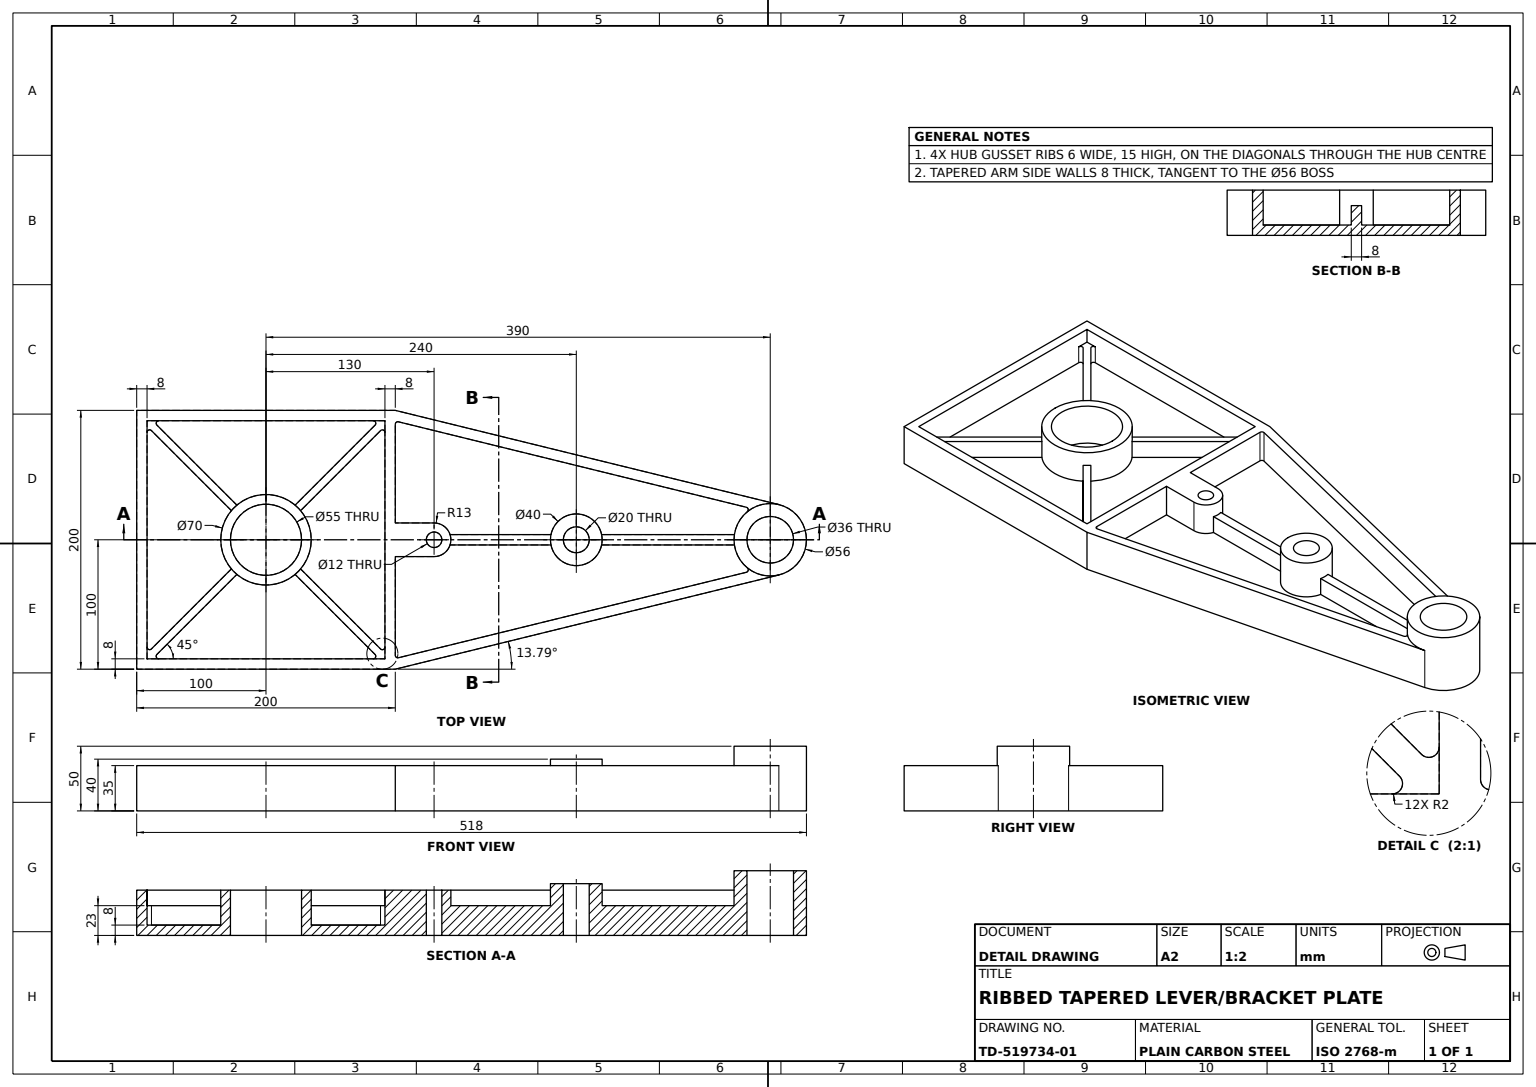
SolidWorks part; units mm, degrees
material "Plain Carbon Steel"
ref_plane "Front Plane" through (0, 0, 0) normal (0, 0, 1) x (1, 0, 0)
ref_plane "Top Plane" through (0, 0, 0) normal (0, 1, 0) x (1, 0, 0)
ref_plane "Right Plane" through (0, 0, 0) normal (1, 0, 0) x (0, 0, -1)
sketch "Base Plate Sketch" plane through (0, 0, 0) normal (0, 1, 0) x (1, 0, 0)
  line L0 (0, 0) -> (0, 390) construction
  line L1 (-100, -100) -> (100, -100)
  line L2 (-100, -100) -> (-100, 100)
  line L4 (100, -100) -> (100, 100)
  line L13 (-100, 100) -> (-27.1931, 396.6735)
  line L14 (100, 100) -> (27.1931, 396.6735)
  line L15 (0, 390) -> (0, 418) construction
  arc A0 (27.1931, 396.6735) -> (-27.1931, 396.6735) centre (0, 390) ccw
  point P0 (0, 0)
  point P6 (0, 0)
  dimension "D3" = 56
  dimension "D1" = 200
  dimension "D2" = 200
  dimension "D4" = 518
  dimension "D5" = 100
extrude "Base Plate 8mm" add sketch "Base Plate Sketch" along normal blind 8
sketch "Perimeter Wall Sketch" plane through (0, 8, 0) normal (0, 1, 0) x (1, 0, 0)
  line L0 (-100, 100) -> (-100, -100) construction
  line L1 (-92, -92) -> (92, -92)
  line L2 (-92, -92) -> (-92, 92)
  line L3 (-92, 92) -> (92, 92)
  line L4 (92, -92) -> (92, 92)
  line L5 (-92, -92) -> (92, 92) construction
  line L6 (-92, 92) -> (92, -92) construction
  line L7 (-100, -100) -> (100, -100) construction
  line L8 (100, -100) -> (100, 100) construction
  line L9 (-100, 100) -> (100, 100)
  line L10 (-100, 100) -> (-100, -100)
  line L11 (-100, -100) -> (100, -100)
  line L12 (100, 100) -> (100, -100)
  line L13 (-100, 100) -> (100, -100) construction
  line L14 (-100, -100) -> (100, 100) construction
  point P0 (0, 0)
  point P10 (0, 0)
  dimension "D1" = 8
  dimension "D2" = 8
extrude "Perimeter Wall" add sketch "Perimeter Wall Sketch" along normal blind 27
sketch "Cross Wall Sketch" plane through (0, 8, 0) normal (0, 1, 0) x (1, 0, 0)
  line L0 (-100, 100) -> (-27.1931, 396.6735)
  line L1 (-27.1931, 396.6735) -> (-100, 100) construction
  line L2 (27.1931, 396.6735) -> (100, 100)
  line L4 (-89.7993, 108) -> (-19.4236, 394.7668)
  line L5 (19.4236, 394.7668) -> (89.7993, 108)
  line L7 (-89.7993, 108) -> (89.7993, 108) construction
  line L8 (-100, 100) -> (100, 100) construction
  line L9 (-100, 92) -> (100, 92)
  line L10 (100, -100) -> (100, 100) construction
  line L11 (-100, 100) -> (-100, -100) construction
  line L12 (-100, 100) -> (-100, 92)
  line L13 (100, 100) -> (-100, 100) construction
  line L14 (-89.7993, 108) -> (-91.7626, 100)
  line L15 (89.7993, 108) -> (91.7626, 100)
  line L16 (-91.7626, 100) -> (91.7626, 100)
  line L17 (-100, 100) -> (100, 100) construction
  line L18 (100, 92) -> (100, 100)
  arc A0 (27.1931, 396.6735) -> (-27.1931, 396.6735) centre (0, 390) ccw
  arc A1 (27.1931, 396.6735) -> (-27.1931, 396.6735) centre (0, 390) ccw construction
  arc A2 (19.4236, 394.7668) -> (-19.4236, 394.7668) centre (0, 390) ccw
  dimension "D2" = 8
  dimension "D1" = 8
  dimension "D3" = 8
extrude "Cross Wall" add sketch "Cross Wall Sketch" along normal up to surface (27 mm away) up to face at (0, 35, 0)
sketch "Tip Boss Sketch" plane through (0, 8, 0) normal (0, 1, 0) x (1, 0, 0)
  circle A0 centre (0, 390) radius 28
  arc A1 (27.1931, 396.6735) -> (-27.1931, 396.6735) centre (0, 390) ccw construction
extrude "Arm Tip Boss" add sketch "Tip Boss Sketch" along normal blind 42
sketch "Arm Pad Sketch" plane through (0, 8, 0) normal (0, 1, 0) x (1, 0, 0)
  line L0 (-13, 130) -> (-13, 100)
  line L1 (13, 130) -> (13, 100)
  line L2 (13, 100) -> (-13, 100)
  line L3 (91.7626, 100) -> (-91.7626, 100) construction
  arc A0 (13, 130) -> (-13, 130) centre (0, 130) ccw
  dimension "D2" = 26
  dimension "D1" = 130
extrude "Arm Pad 130x26" add sketch "Arm Pad Sketch" along normal up to surface (27 mm away) up to face at (0, 35, 0)
sketch "Hub Boss Sketch" plane through (0, 8, 0) normal (0, 1, 0) x (1, 0, 0)
  circle A0 centre (0, 0) radius 35
  dimension "D1" = 70
extrude "Hub Boss Ø70" add sketch "Hub Boss Sketch" along normal blind 27
sketch "Mid Boss Sketch" plane through (0, 8, 0) normal (0, 1, 0) x (1, 0, 0)
  circle A0 centre (0, 240) radius 20
  dimension "D1" = 40
  dimension "D2" = 240
extrude "Mid Arm Boss Ø40" add sketch "Mid Boss Sketch" along normal blind 32
sketch "Hub Ribs Sketch" plane through (0, 8, 0) normal (0, 1, 0) x (1, 0, 0)
  line L0 (89.7946, 94.0219) -> (22.5446, 26.772)
  line L1 (94.0372, 89.7793) -> (26.786, 22.528)
  line L2 (89.7946, 94.0219) -> (94.0372, 89.7793)
  line L3 (94.0219, -89.7946) -> (26.772, -22.5446)
  line L4 (-94.0219, 89.7946) -> (-26.772, 22.5446)
  line L5 (89.7793, -94.0372) -> (22.528, -26.786)
  line L6 (94.0219, -89.7946) -> (89.7793, -94.0372)
  line L7 (-89.7946, -94.0219) -> (-22.5446, -26.772)
  line L8 (-89.7793, 94.0372) -> (-22.528, 26.786)
  line L9 (-94.0372, -89.7793) -> (-26.786, -22.528)
  line L10 (-89.7946, -94.0219) -> (-94.0372, -89.7793)
  line L11 (92, -92) -> (92, 92) construction
  line L12 (-94.0219, 89.7946) -> (-89.7793, 94.0372)
  circle A0 centre (0, 0) radius 35 construction
  arc A1 (-26.772, 22.5446) -> (-26.786, -22.528) centre (0, 0) ccw
  arc A2 (22.5446, 26.772) -> (-22.528, 26.786) centre (0, 0) ccw
  arc A3 (26.772, -22.5446) -> (26.786, 22.528) centre (0, 0) ccw
  arc A4 (-22.5446, -26.772) -> (22.528, -26.786) centre (0, 0) ccw
  dimension "D1" = 6
  dimension "D3" = 2.0219
  dimension "D4" = 2.0372
  dimension "D5" = 2.2054
  dimension "D2" = 4
extrude "Hub Gusset Ribs 4x" add sketch "Hub Ribs Sketch" along normal blind 15
fillet "Wall and Rib Fillets R2" radius 2 12 edges at (91.7626, 21.5, -100) (87.7421, 15.5, 92) (92, 15.5, 87.7726) (87.7726, 15.5, -92) (92, 15.5, -87.7421) (-91.7626, 21.5, -100) (-92, 15.5, 87.7421) (-87.7726, 15.5, 92) (-92, 15.5, -87.7726) (-87.7421, 15.5, -92) (24.0941, 21.5, -375.7356) (-24.0941, 21.5, -375.7356)
sketch "Arm Ribs Sketch" plane through (0, 8, 0) normal (0, 1, 0) x (1, 0, 0)
  line L0 (-4, 100.8496) -> (4, 100.8496)
  line L2 (4, 100.8496) -> (4, 366.4206)
  line L3 (-4, 100.8496) -> (-4, 366.4206)
  line L4 (-4, 366.4206) -> (4, 366.4206)
  point P1 (0, 366.4206)
  point P4 (0, 100.8496)
  dimension "D1" = 87.1548
  dimension "D2" = 263.9439
  dimension "D3" = 1.627
extrude "Arm Gusset Ribs" add sketch "Arm Ribs Sketch" along normal blind 15
sketch "Boss Bores Sketch" plane through (0, 0, 0) normal (0, -1, 0) x (1, 0, 0)
  circle A0 centre (0, 0) radius 27.5
  circle A1 centre (0, -130) radius 6
  arc A2 (-13, -130) -> (13, -130) centre (0, -130) ccw construction
  arc A4 (26.786, -22.528) -> (26.772, 22.5446) centre (0, 0) ccw construction
  circle A5 centre (0, -240) radius 10
  circle A6 centre (0, -390) radius 18
  dimension "D1" = 55
  dimension "D2" = 12
  dimension "D3" = 20
  dimension "D4" = 36
extrude "Boss Bores" cut sketch "Boss Bores Sketch" against normal through all
